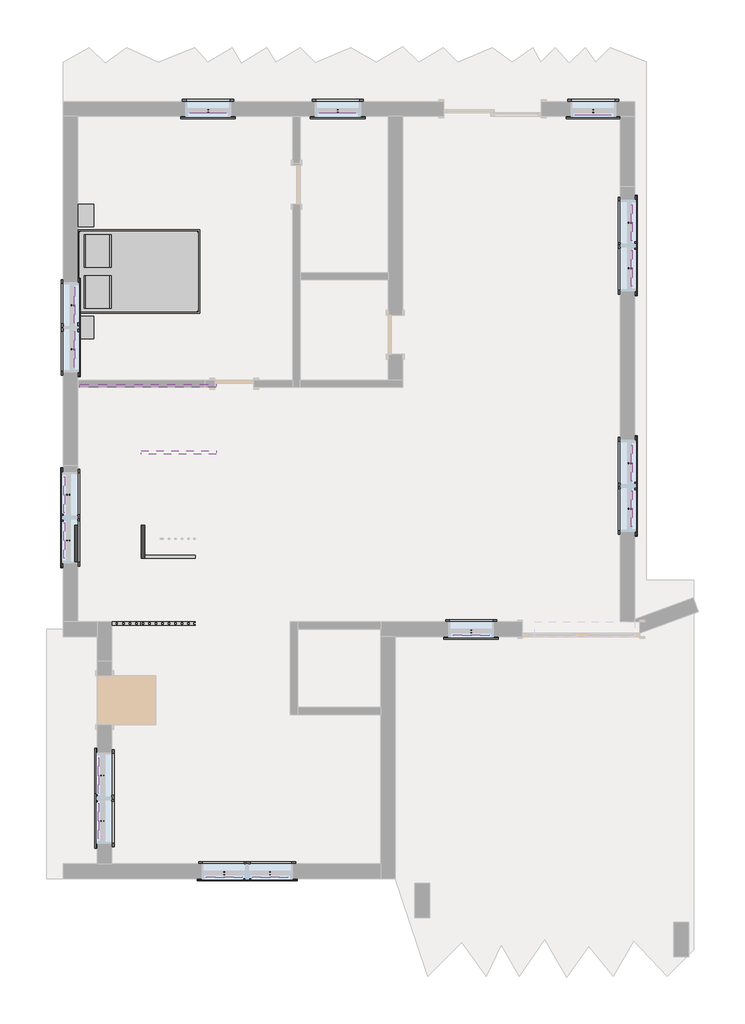
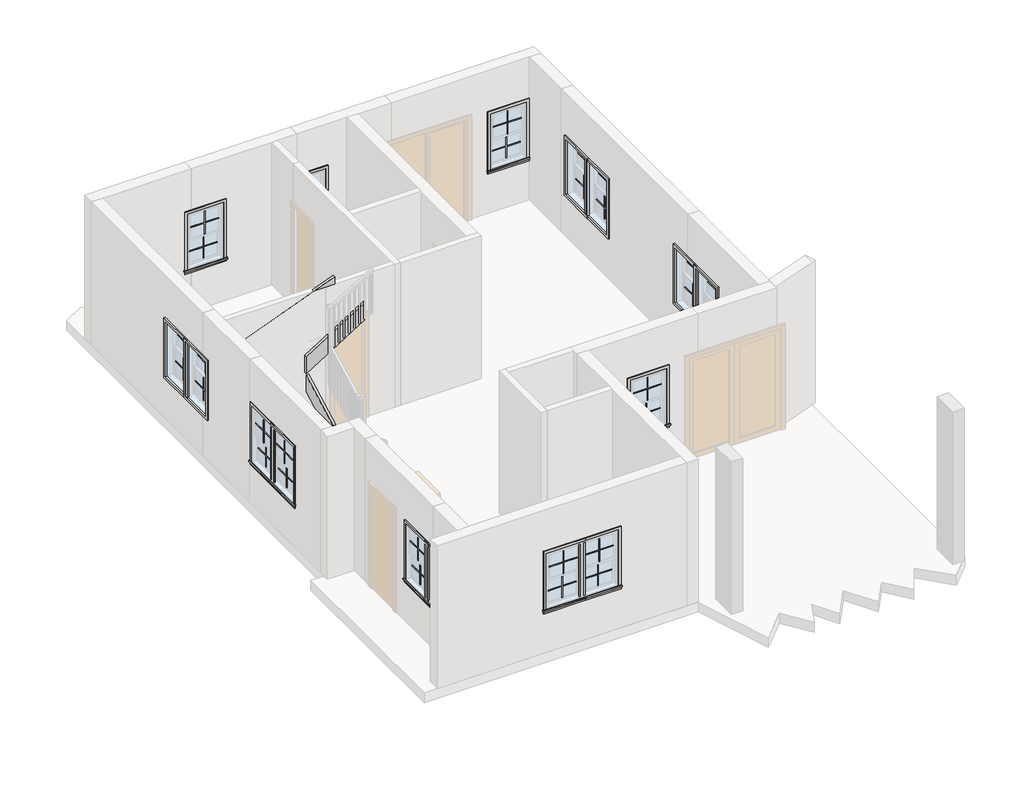
# One storey, part 3 of 3: 64 proxies, 6 members, 1 furniture element.
"""IFC4 building model written with IfcOpenShell, lengths in millimetres."""

from ifc_helpers import new_model, si_unit, frame, origin, place, context, project, spatial, polyline, outline, extrude, transform, mapped, element, save
from components import muntin_pattern_2x2_muntin_pattern_2x2_5f474966, trim_window_exterior_flat_with_sill_68241f6a, trim_window_interior_flat_picture_frame_d3d93820, modern_beds_1593_1300_x_1900_cc95cf5d

model = new_model("IFC4")

# Units and contexts
model_context = context("Model", 3, world=origin())
ifc_project = project(units=[si_unit("LENGTHUNIT", "METRE", prefix="MILLI")], contexts=[model_context])

# Site, building, storey
site = spatial("IfcSite", under=ifc_project)
building = spatial("IfcBuilding", under=site)
storey = spatial("IfcBuildingStorey", under=building, Elevation=3200.4)

# Proxies
placement = place(None, origin())
muntin_pattern_2x2_muntin_pattern_2x2_shape = muntin_pattern_2x2_muntin_pattern_2x2_5f474966(model_context)
element("IfcBuildingElementProxy", 1, Name="Muntin Pattern_2x2 : Muntin Pattern_2x2", ObjectType="Muntin Pattern_2x2 : Muntin Pattern_2x2", at=placement, inside=storey, context=model_context, shape_type="MappedRepresentation", body=[
    mapped(muntin_pattern_2x2_muntin_pattern_2x2_shape, transform((-20215.5750314, 12584.9473147, 4721.225), x_axis=(-1.0, 0.0, 0.0), y_axis=(0.0, -1.0, 0.0), z_axis=(0.0, 0.0, 1.0))),
])
element("IfcBuildingElementProxy", 2, Name="Muntin Pattern_2x2 : Muntin Pattern_2x2", ObjectType="Muntin Pattern_2x2 : Muntin Pattern_2x2", at=placement, inside=storey, context=model_context, shape_type="MappedRepresentation", body=[
    mapped(muntin_pattern_2x2_muntin_pattern_2x2_shape, transform((-20215.5750314, 12629.3973147, 4191.0), x_axis=(-1.0, 0.0, 0.0), y_axis=(0.0, -1.0, 0.0), z_axis=(0.0, 0.0, 1.0))),
])
element("IfcBuildingElementProxy", 3, Name="Muntin Pattern_2x2 : Muntin Pattern_2x2", ObjectType="Muntin Pattern_2x2 : Muntin Pattern_2x2", at=placement, inside=storey, context=model_context, shape_type="MappedRepresentation", body=[
    mapped(muntin_pattern_2x2_muntin_pattern_2x2_shape, transform((-14208.4750314, 12584.9473147, 4721.225), x_axis=(-1.0, 0.0, 0.0), y_axis=(0.0, -1.0, 0.0), z_axis=(0.0, 0.0, 1.0))),
])
element("IfcBuildingElementProxy", 4, Name="Muntin Pattern_2x2 : Muntin Pattern_2x2", ObjectType="Muntin Pattern_2x2 : Muntin Pattern_2x2", at=placement, inside=storey, context=model_context, shape_type="MappedRepresentation", body=[
    mapped(muntin_pattern_2x2_muntin_pattern_2x2_shape, transform((-14208.4750314, 12629.3973147, 4191.0), x_axis=(-1.0, 0.0, 0.0), y_axis=(0.0, -1.0, 0.0), z_axis=(0.0, 0.0, 1.0))),
])
element("IfcBuildingElementProxy", 5, Name="Muntin Pattern_2x2 : Muntin Pattern_2x2", ObjectType="Muntin Pattern_2x2 : Muntin Pattern_2x2", at=placement, inside=storey, context=model_context, shape_type="MappedRepresentation", body=[
    mapped(muntin_pattern_2x2_muntin_pattern_2x2_shape, transform((-13595.7000314, 10888.3098201, 4721.225), x_axis=(0.0, -1.0, 0.0), y_axis=(1.0, 0.0, 0.0), z_axis=(0.0, 0.0, 1.0))),
])
element("IfcBuildingElementProxy", 6, Name="Muntin Pattern_2x2 : Muntin Pattern_2x2", ObjectType="Muntin Pattern_2x2 : Muntin Pattern_2x2", at=placement, inside=storey, context=model_context, shape_type="MappedRepresentation", body=[
    mapped(muntin_pattern_2x2_muntin_pattern_2x2_shape, transform((-13640.1500314, 10888.3098201, 4191.0), x_axis=(0.0, -1.0, 0.0), y_axis=(1.0, 0.0, 0.0), z_axis=(0.0, 0.0, 1.0))),
])
element("IfcBuildingElementProxy", 7, Name="Muntin Pattern_2x2 : Muntin Pattern_2x2", ObjectType="Muntin Pattern_2x2 : Muntin Pattern_2x2", at=placement, inside=storey, context=model_context, shape_type="MappedRepresentation", body=[
    mapped(muntin_pattern_2x2_muntin_pattern_2x2_shape, transform((-13595.7000314, 10177.1098201, 4721.225), x_axis=(0.0, -1.0, 0.0), y_axis=(1.0, 0.0, 0.0), z_axis=(0.0, 0.0, 1.0))),
])
element("IfcBuildingElementProxy", 8, Name="Muntin Pattern_2x2 : Muntin Pattern_2x2", ObjectType="Muntin Pattern_2x2 : Muntin Pattern_2x2", at=placement, inside=storey, context=model_context, shape_type="MappedRepresentation", body=[
    mapped(muntin_pattern_2x2_muntin_pattern_2x2_shape, transform((-13640.1500314, 10177.1098201, 4191.0), x_axis=(0.0, -1.0, 0.0), y_axis=(1.0, 0.0, 0.0), z_axis=(0.0, 0.0, 1.0))),
])
element("IfcBuildingElementProxy", 9, Name="Muntin Pattern_2x2 : Muntin Pattern_2x2", ObjectType="Muntin Pattern_2x2 : Muntin Pattern_2x2", at=placement, inside=storey, context=model_context, shape_type="MappedRepresentation", body=[
    mapped(muntin_pattern_2x2_muntin_pattern_2x2_shape, transform((-13595.7000314, 7139.8223646, 4721.225), x_axis=(0.0, -1.0, 0.0), y_axis=(1.0, 0.0, 0.0), z_axis=(0.0, 0.0, 1.0))),
])
element("IfcBuildingElementProxy", 10, Name="Muntin Pattern_2x2 : Muntin Pattern_2x2", ObjectType="Muntin Pattern_2x2 : Muntin Pattern_2x2", at=placement, inside=storey, context=model_context, shape_type="MappedRepresentation", body=[
    mapped(muntin_pattern_2x2_muntin_pattern_2x2_shape, transform((-13640.1500314, 7139.8223646, 4191.0), x_axis=(0.0, -1.0, 0.0), y_axis=(1.0, 0.0, 0.0), z_axis=(0.0, 0.0, 1.0))),
])
element("IfcBuildingElementProxy", 11, Name="Muntin Pattern_2x2 : Muntin Pattern_2x2", ObjectType="Muntin Pattern_2x2 : Muntin Pattern_2x2", at=placement, inside=storey, context=model_context, shape_type="MappedRepresentation", body=[
    mapped(muntin_pattern_2x2_muntin_pattern_2x2_shape, transform((-13595.7000314, 6428.6223646, 4721.225), x_axis=(0.0, -1.0, 0.0), y_axis=(1.0, 0.0, 0.0), z_axis=(0.0, 0.0, 1.0))),
])
element("IfcBuildingElementProxy", 12, Name="Muntin Pattern_2x2 : Muntin Pattern_2x2", ObjectType="Muntin Pattern_2x2 : Muntin Pattern_2x2", at=placement, inside=storey, context=model_context, shape_type="MappedRepresentation", body=[
    mapped(muntin_pattern_2x2_muntin_pattern_2x2_shape, transform((-13640.1500314, 6428.6223646, 4191.0), x_axis=(0.0, -1.0, 0.0), y_axis=(1.0, 0.0, 0.0), z_axis=(0.0, 0.0, 1.0))),
])
element("IfcBuildingElementProxy", 13, Name="Muntin Pattern_2x2 : Muntin Pattern_2x2", ObjectType="Muntin Pattern_2x2 : Muntin Pattern_2x2", at=placement, inside=storey, context=model_context, shape_type="MappedRepresentation", body=[
    mapped(muntin_pattern_2x2_muntin_pattern_2x2_shape, transform((-19961.4931686, 697.7473646, 4721.225), x_axis=(-1.0, 0.0, 0.0), y_axis=(0.0, -1.0, 0.0), z_axis=(0.0, 0.0, 1.0))),
])
element("IfcBuildingElementProxy", 14, Name="Muntin Pattern_2x2 : Muntin Pattern_2x2", ObjectType="Muntin Pattern_2x2 : Muntin Pattern_2x2", at=placement, inside=storey, context=model_context, shape_type="MappedRepresentation", body=[
    mapped(muntin_pattern_2x2_muntin_pattern_2x2_shape, transform((-19961.4931686, 742.1973646, 4191.0), x_axis=(-1.0, 0.0, 0.0), y_axis=(0.0, -1.0, 0.0), z_axis=(0.0, 0.0, 1.0))),
])
element("IfcBuildingElementProxy", 15, Name="Muntin Pattern_2x2 : Muntin Pattern_2x2", ObjectType="Muntin Pattern_2x2 : Muntin Pattern_2x2", at=placement, inside=storey, context=model_context, shape_type="MappedRepresentation", body=[
    mapped(muntin_pattern_2x2_muntin_pattern_2x2_shape, transform((-19250.2931686, 697.7473646, 4721.225), x_axis=(-1.0, 0.0, 0.0), y_axis=(0.0, -1.0, 0.0), z_axis=(0.0, 0.0, 1.0))),
])
element("IfcBuildingElementProxy", 16, Name="Muntin Pattern_2x2 : Muntin Pattern_2x2", ObjectType="Muntin Pattern_2x2 : Muntin Pattern_2x2", at=placement, inside=storey, context=model_context, shape_type="MappedRepresentation", body=[
    mapped(muntin_pattern_2x2_muntin_pattern_2x2_shape, transform((-19250.2931686, 742.1973646, 4191.0), x_axis=(-1.0, 0.0, 0.0), y_axis=(0.0, -1.0, 0.0), z_axis=(0.0, 0.0, 1.0))),
])
element("IfcBuildingElementProxy", 17, Name="Muntin Pattern_2x2 : Muntin Pattern_2x2", ObjectType="Muntin Pattern_2x2 : Muntin Pattern_2x2", at=placement, inside=storey, context=model_context, shape_type="MappedRepresentation", body=[
    mapped(muntin_pattern_2x2_muntin_pattern_2x2_shape, transform((-21907.8500314, 2269.3723646, 4721.225), x_axis=(0.0, 1.0, 0.0), y_axis=(-1.0, 0.0, 0.0), z_axis=(0.0, 0.0, 1.0))),
])
element("IfcBuildingElementProxy", 18, Name="Muntin Pattern_2x2 : Muntin Pattern_2x2", ObjectType="Muntin Pattern_2x2 : Muntin Pattern_2x2", at=placement, inside=storey, context=model_context, shape_type="MappedRepresentation", body=[
    mapped(muntin_pattern_2x2_muntin_pattern_2x2_shape, transform((-21863.4000314, 2269.3723646, 4191.0), x_axis=(0.0, 1.0, 0.0), y_axis=(-1.0, 0.0, 0.0), z_axis=(0.0, 0.0, 1.0))),
])
element("IfcBuildingElementProxy", 19, Name="Muntin Pattern_2x2 : Muntin Pattern_2x2", ObjectType="Muntin Pattern_2x2 : Muntin Pattern_2x2", at=placement, inside=storey, context=model_context, shape_type="MappedRepresentation", body=[
    mapped(muntin_pattern_2x2_muntin_pattern_2x2_shape, transform((-21907.8500314, 1558.1723646, 4721.225), x_axis=(0.0, 1.0, 0.0), y_axis=(-1.0, 0.0, 0.0), z_axis=(0.0, 0.0, 1.0))),
])
element("IfcBuildingElementProxy", 20, Name="Muntin Pattern_2x2 : Muntin Pattern_2x2", ObjectType="Muntin Pattern_2x2 : Muntin Pattern_2x2", at=placement, inside=storey, context=model_context, shape_type="MappedRepresentation", body=[
    mapped(muntin_pattern_2x2_muntin_pattern_2x2_shape, transform((-21863.4000314, 1558.1723646, 4191.0), x_axis=(0.0, 1.0, 0.0), y_axis=(-1.0, 0.0, 0.0), z_axis=(0.0, 0.0, 1.0))),
])
element("IfcBuildingElementProxy", 21, Name="Muntin Pattern_2x2 : Muntin Pattern_2x2", ObjectType="Muntin Pattern_2x2 : Muntin Pattern_2x2", at=placement, inside=storey, context=model_context, shape_type="MappedRepresentation", body=[
    mapped(muntin_pattern_2x2_muntin_pattern_2x2_shape, transform((-22441.2502061, 6644.5223643, 4721.225), x_axis=(0.0, 1.0, 0.0), y_axis=(-1.0, 0.0, 0.0), z_axis=(0.0, 0.0, 1.0))),
])
element("IfcBuildingElementProxy", 22, Name="Muntin Pattern_2x2 : Muntin Pattern_2x2", ObjectType="Muntin Pattern_2x2 : Muntin Pattern_2x2", at=placement, inside=storey, context=model_context, shape_type="MappedRepresentation", body=[
    mapped(muntin_pattern_2x2_muntin_pattern_2x2_shape, transform((-22396.8002061, 6644.5223643, 4191.0), x_axis=(0.0, 1.0, 0.0), y_axis=(-1.0, 0.0, 0.0), z_axis=(0.0, 0.0, 1.0))),
])
element("IfcBuildingElementProxy", 23, Name="Muntin Pattern_2x2 : Muntin Pattern_2x2", ObjectType="Muntin Pattern_2x2 : Muntin Pattern_2x2", at=placement, inside=storey, context=model_context, shape_type="MappedRepresentation", body=[
    mapped(muntin_pattern_2x2_muntin_pattern_2x2_shape, transform((-22441.2502061, 5933.3223643, 4721.225), x_axis=(0.0, 1.0, 0.0), y_axis=(-1.0, 0.0, 0.0), z_axis=(0.0, 0.0, 1.0))),
])
element("IfcBuildingElementProxy", 24, Name="Muntin Pattern_2x2 : Muntin Pattern_2x2", ObjectType="Muntin Pattern_2x2 : Muntin Pattern_2x2", at=placement, inside=storey, context=model_context, shape_type="MappedRepresentation", body=[
    mapped(muntin_pattern_2x2_muntin_pattern_2x2_shape, transform((-22396.8002061, 5933.3223643, 4191.0), x_axis=(0.0, 1.0, 0.0), y_axis=(-1.0, 0.0, 0.0), z_axis=(0.0, 0.0, 1.0))),
])
element("IfcBuildingElementProxy", 25, Name="Muntin Pattern_2x2 : Muntin Pattern_2x2", ObjectType="Muntin Pattern_2x2 : Muntin Pattern_2x2", at=placement, inside=storey, context=model_context, shape_type="MappedRepresentation", body=[
    mapped(muntin_pattern_2x2_muntin_pattern_2x2_shape, transform((-22282.5000314, 9599.539033, 4721.225), x_axis=(0.0, -1.0, 0.0), y_axis=(1.0, 0.0, 0.0), z_axis=(0.0, 0.0, 1.0))),
])
element("IfcBuildingElementProxy", 26, Name="Muntin Pattern_2x2 : Muntin Pattern_2x2", ObjectType="Muntin Pattern_2x2 : Muntin Pattern_2x2", at=placement, inside=storey, context=model_context, shape_type="MappedRepresentation", body=[
    mapped(muntin_pattern_2x2_muntin_pattern_2x2_shape, transform((-22326.9500314, 9599.539033, 4191.0), x_axis=(0.0, -1.0, 0.0), y_axis=(1.0, 0.0, 0.0), z_axis=(0.0, 0.0, 1.0))),
])
element("IfcBuildingElementProxy", 27, Name="Muntin Pattern_2x2 : Muntin Pattern_2x2", ObjectType="Muntin Pattern_2x2 : Muntin Pattern_2x2", at=placement, inside=storey, context=model_context, shape_type="MappedRepresentation", body=[
    mapped(muntin_pattern_2x2_muntin_pattern_2x2_shape, transform((-22282.5000314, 8913.739033, 4721.225), x_axis=(0.0, -1.0, 0.0), y_axis=(1.0, 0.0, 0.0), z_axis=(0.0, 0.0, 1.0))),
])
element("IfcBuildingElementProxy", 28, Name="Muntin Pattern_2x2 : Muntin Pattern_2x2", ObjectType="Muntin Pattern_2x2 : Muntin Pattern_2x2", at=placement, inside=storey, context=model_context, shape_type="MappedRepresentation", body=[
    mapped(muntin_pattern_2x2_muntin_pattern_2x2_shape, transform((-22326.9500314, 8913.739033, 4191.0), x_axis=(0.0, -1.0, 0.0), y_axis=(1.0, 0.0, 0.0), z_axis=(0.0, 0.0, 1.0))),
])
element("IfcBuildingElementProxy", 29, Name="Muntin Pattern_2x2 : Muntin Pattern_2x2", ObjectType="Muntin Pattern_2x2 : Muntin Pattern_2x2", at=placement, inside=storey, context=model_context, shape_type="MappedRepresentation", body=[
    mapped(muntin_pattern_2x2_muntin_pattern_2x2_shape, transform((-18193.8494379, 12584.9473147, 4721.225), x_axis=(-1.0, 0.0, 0.0), y_axis=(0.0, -1.0, 0.0), z_axis=(0.0, 0.0, 1.0))),
])
element("IfcBuildingElementProxy", 30, Name="Muntin Pattern_2x2 : Muntin Pattern_2x2", ObjectType="Muntin Pattern_2x2 : Muntin Pattern_2x2", at=placement, inside=storey, context=model_context, shape_type="MappedRepresentation", body=[
    mapped(muntin_pattern_2x2_muntin_pattern_2x2_shape, transform((-18193.8494379, 12629.3973147, 4191.0), x_axis=(-1.0, 0.0, 0.0), y_axis=(0.0, -1.0, 0.0), z_axis=(0.0, 0.0, 1.0))),
])
element("IfcBuildingElementProxy", 31, Name="Muntin Pattern_2x2 : Muntin Pattern_2x2", ObjectType="Muntin Pattern_2x2 : Muntin Pattern_2x2", at=placement, inside=storey, context=model_context, shape_type="MappedRepresentation", body=[
    mapped(muntin_pattern_2x2_muntin_pattern_2x2_shape, transform((-16113.4750314, 4469.6473722, 4721.225), x_axis=(-1.0, 0.0, 0.0), y_axis=(0.0, -1.0, 0.0), z_axis=(0.0, 0.0, 1.0))),
])
element("IfcBuildingElementProxy", 32, Name="Muntin Pattern_2x2 : Muntin Pattern_2x2", ObjectType="Muntin Pattern_2x2 : Muntin Pattern_2x2", at=placement, inside=storey, context=model_context, shape_type="MappedRepresentation", body=[
    mapped(muntin_pattern_2x2_muntin_pattern_2x2_shape, transform((-16113.4750314, 4514.0973722, 4191.0), x_axis=(-1.0, 0.0, 0.0), y_axis=(0.0, -1.0, 0.0), z_axis=(0.0, 0.0, 1.0))),
])
trim_window_exterior_flat_with_sill_shape = trim_window_exterior_flat_with_sill_68241f6a(model_context)
element("IfcBuildingElementProxy", 33, Name="Trim-Window-Exterior-Flat : with Sill", ObjectType="Trim-Window-Exterior-Flat : with Sill", at=placement, inside=storey, context=model_context, shape_type="MappedRepresentation", body=[
    mapped(trim_window_exterior_flat_with_sill_shape, transform((-20215.5750314, 12550.0223147, 5283.2), x_axis=(1.0, 0.0, 0.0), y_axis=(0.0, 0.0, 1.0), z_axis=(0.0, -1.0, 0.0))),
])
element("IfcBuildingElementProxy", 34, Name="Trim-Window-Exterior-Flat : with Sill", ObjectType="Trim-Window-Exterior-Flat : with Sill", at=placement, inside=storey, context=model_context, shape_type="MappedRepresentation", body=[
    mapped(trim_window_exterior_flat_with_sill_shape, transform((-14208.4750314, 12550.0223147, 5283.2), x_axis=(1.0, 0.0, 0.0), y_axis=(0.0, 0.0, 1.0), z_axis=(0.0, -1.0, 0.0))),
])
element("IfcBuildingElementProxy", 35, Name="Trim-Window-Exterior-Flat : with Sill", ObjectType="Trim-Window-Exterior-Flat : with Sill", at=placement, inside=storey, context=model_context, shape_type="MappedRepresentation", body=[
    mapped(trim_window_exterior_flat_with_sill_shape, transform((-13560.7750314, 10888.3098201, 5283.2), x_axis=(0.0, 1.0, 0.0), y_axis=(0.0, 0.0, 1.0), z_axis=(1.0, 0.0, 0.0))),
])
element("IfcBuildingElementProxy", 36, Name="Trim-Window-Exterior-Flat : with Sill", ObjectType="Trim-Window-Exterior-Flat : with Sill", at=placement, inside=storey, context=model_context, shape_type="MappedRepresentation", body=[
    mapped(trim_window_exterior_flat_with_sill_shape, transform((-13560.7750314, 10177.1098201, 5283.2), x_axis=(0.0, 1.0, 0.0), y_axis=(0.0, 0.0, 1.0), z_axis=(1.0, 0.0, 0.0))),
])
element("IfcBuildingElementProxy", 37, Name="Trim-Window-Exterior-Flat : with Sill", ObjectType="Trim-Window-Exterior-Flat : with Sill", at=placement, inside=storey, context=model_context, shape_type="MappedRepresentation", body=[
    mapped(trim_window_exterior_flat_with_sill_shape, transform((-13560.7750314, 7139.8223646, 5283.2), x_axis=(0.0, 1.0, 0.0), y_axis=(0.0, 0.0, 1.0), z_axis=(1.0, 0.0, 0.0))),
])
element("IfcBuildingElementProxy", 38, Name="Trim-Window-Exterior-Flat : with Sill", ObjectType="Trim-Window-Exterior-Flat : with Sill", at=placement, inside=storey, context=model_context, shape_type="MappedRepresentation", body=[
    mapped(trim_window_exterior_flat_with_sill_shape, transform((-13560.7750314, 6428.6223646, 5283.2), x_axis=(0.0, 1.0, 0.0), y_axis=(0.0, 0.0, 1.0), z_axis=(1.0, 0.0, 0.0))),
])
element("IfcBuildingElementProxy", 39, Name="Trim-Window-Exterior-Flat : with Sill", ObjectType="Trim-Window-Exterior-Flat : with Sill", at=placement, inside=storey, context=model_context, shape_type="MappedRepresentation", body=[
    mapped(trim_window_exterior_flat_with_sill_shape, transform((-19961.4931686, 662.8223646, 5283.2), x_axis=(1.0, 0.0, 0.0), y_axis=(0.0, 0.0, 1.0), z_axis=(0.0, -1.0, 0.0))),
])
element("IfcBuildingElementProxy", 40, Name="Trim-Window-Exterior-Flat : with Sill", ObjectType="Trim-Window-Exterior-Flat : with Sill", at=placement, inside=storey, context=model_context, shape_type="MappedRepresentation", body=[
    mapped(trim_window_exterior_flat_with_sill_shape, transform((-19250.2931686, 662.8223646, 5283.2), x_axis=(1.0, 0.0, 0.0), y_axis=(0.0, 0.0, 1.0), z_axis=(0.0, -1.0, 0.0))),
])
element("IfcBuildingElementProxy", 41, Name="Trim-Window-Exterior-Flat : with Sill", ObjectType="Trim-Window-Exterior-Flat : with Sill", at=placement, inside=storey, context=model_context, shape_type="MappedRepresentation", body=[
    mapped(trim_window_exterior_flat_with_sill_shape, transform((-21942.7750314, 2269.3723646, 5283.2), x_axis=(0.0, -1.0, 0.0), y_axis=(0.0, 0.0, 1.0), z_axis=(-1.0, 0.0, 0.0))),
])
element("IfcBuildingElementProxy", 42, Name="Trim-Window-Exterior-Flat : with Sill", ObjectType="Trim-Window-Exterior-Flat : with Sill", at=placement, inside=storey, context=model_context, shape_type="MappedRepresentation", body=[
    mapped(trim_window_exterior_flat_with_sill_shape, transform((-21942.7750314, 1558.1723646, 5283.2), x_axis=(0.0, -1.0, 0.0), y_axis=(0.0, 0.0, 1.0), z_axis=(-1.0, 0.0, 0.0))),
])
element("IfcBuildingElementProxy", 43, Name="Trim-Window-Exterior-Flat : with Sill", ObjectType="Trim-Window-Exterior-Flat : with Sill", at=placement, inside=storey, context=model_context, shape_type="MappedRepresentation", body=[
    mapped(trim_window_exterior_flat_with_sill_shape, transform((-22476.1752061, 6644.5223643, 5283.2), x_axis=(0.0, -1.0, 0.0), y_axis=(0.0, 0.0, 1.0), z_axis=(-1.0, 0.0, 0.0))),
])
element("IfcBuildingElementProxy", 44, Name="Trim-Window-Exterior-Flat : with Sill", ObjectType="Trim-Window-Exterior-Flat : with Sill", at=placement, inside=storey, context=model_context, shape_type="MappedRepresentation", body=[
    mapped(trim_window_exterior_flat_with_sill_shape, transform((-22476.1752061, 5933.3223643, 5283.2), x_axis=(0.0, -1.0, 0.0), y_axis=(0.0, 0.0, 1.0), z_axis=(-1.0, 0.0, 0.0))),
])
element("IfcBuildingElementProxy", 45, Name="Trim-Window-Exterior-Flat : with Sill", ObjectType="Trim-Window-Exterior-Flat : with Sill", at=placement, inside=storey, context=model_context, shape_type="MappedRepresentation", body=[
    mapped(trim_window_exterior_flat_with_sill_shape, transform((-22247.5750314, 9599.539033, 5283.2), x_axis=(0.0, 1.0, 0.0), y_axis=(0.0, 0.0, 1.0), z_axis=(1.0, 0.0, 0.0))),
])
element("IfcBuildingElementProxy", 46, Name="Trim-Window-Exterior-Flat : with Sill", ObjectType="Trim-Window-Exterior-Flat : with Sill", at=placement, inside=storey, context=model_context, shape_type="MappedRepresentation", body=[
    mapped(trim_window_exterior_flat_with_sill_shape, transform((-22247.5750314, 8913.739033, 5283.2), x_axis=(0.0, 1.0, 0.0), y_axis=(0.0, 0.0, 1.0), z_axis=(1.0, 0.0, 0.0))),
])
element("IfcBuildingElementProxy", 47, Name="Trim-Window-Exterior-Flat : with Sill", ObjectType="Trim-Window-Exterior-Flat : with Sill", at=placement, inside=storey, context=model_context, shape_type="MappedRepresentation", body=[
    mapped(trim_window_exterior_flat_with_sill_shape, transform((-18193.8494379, 12550.0223147, 5283.2), x_axis=(1.0, 0.0, 0.0), y_axis=(0.0, 0.0, 1.0), z_axis=(0.0, -1.0, 0.0))),
])
element("IfcBuildingElementProxy", 48, Name="Trim-Window-Exterior-Flat : with Sill", ObjectType="Trim-Window-Exterior-Flat : with Sill", at=placement, inside=storey, context=model_context, shape_type="MappedRepresentation", body=[
    mapped(trim_window_exterior_flat_with_sill_shape, transform((-16113.4750314, 4434.7223722, 5283.2), x_axis=(1.0, 0.0, 0.0), y_axis=(0.0, 0.0, 1.0), z_axis=(0.0, -1.0, 0.0))),
])
trim_window_interior_flat_picture_frame_shape = trim_window_interior_flat_picture_frame_d3d93820(model_context)
element("IfcBuildingElementProxy", 49, Name="Trim-Window-Interior-Flat : Picture Frame", ObjectType="Trim-Window-Interior-Flat : Picture Frame", at=placement, inside=storey, context=model_context, shape_type="MappedRepresentation", body=[
    mapped(trim_window_interior_flat_picture_frame_shape, transform((-20215.5750314, 12778.6223147, 5283.2), x_axis=(-1.0, 0.0, 0.0), y_axis=(0.0, 0.0, 1.0), z_axis=(0.0, 1.0, 0.0))),
])
element("IfcBuildingElementProxy", 50, Name="Trim-Window-Interior-Flat : Picture Frame", ObjectType="Trim-Window-Interior-Flat : Picture Frame", at=placement, inside=storey, context=model_context, shape_type="MappedRepresentation", body=[
    mapped(trim_window_interior_flat_picture_frame_shape, transform((-14208.4750314, 12778.6223147, 5283.2), x_axis=(-1.0, 0.0, 0.0), y_axis=(0.0, 0.0, 1.0), z_axis=(0.0, 1.0, 0.0))),
])
element("IfcBuildingElementProxy", 51, Name="Trim-Window-Interior-Flat : Picture Frame", ObjectType="Trim-Window-Interior-Flat : Picture Frame", at=placement, inside=storey, context=model_context, shape_type="MappedRepresentation", body=[
    mapped(trim_window_interior_flat_picture_frame_shape, transform((-13789.3750314, 10888.3098201, 5283.2), x_axis=(0.0, -1.0, 0.0), y_axis=(0.0, 0.0, 1.0), z_axis=(-1.0, 0.0, 0.0))),
])
element("IfcBuildingElementProxy", 52, Name="Trim-Window-Interior-Flat : Picture Frame", ObjectType="Trim-Window-Interior-Flat : Picture Frame", at=placement, inside=storey, context=model_context, shape_type="MappedRepresentation", body=[
    mapped(trim_window_interior_flat_picture_frame_shape, transform((-13789.3750314, 10177.1098201, 5283.2), x_axis=(0.0, -1.0, 0.0), y_axis=(0.0, 0.0, 1.0), z_axis=(-1.0, 0.0, 0.0))),
])
element("IfcBuildingElementProxy", 53, Name="Trim-Window-Interior-Flat : Picture Frame", ObjectType="Trim-Window-Interior-Flat : Picture Frame", at=placement, inside=storey, context=model_context, shape_type="MappedRepresentation", body=[
    mapped(trim_window_interior_flat_picture_frame_shape, transform((-13789.3750314, 7139.8223646, 5283.2), x_axis=(0.0, -1.0, 0.0), y_axis=(0.0, 0.0, 1.0), z_axis=(-1.0, 0.0, 0.0))),
])
element("IfcBuildingElementProxy", 54, Name="Trim-Window-Interior-Flat : Picture Frame", ObjectType="Trim-Window-Interior-Flat : Picture Frame", at=placement, inside=storey, context=model_context, shape_type="MappedRepresentation", body=[
    mapped(trim_window_interior_flat_picture_frame_shape, transform((-13789.3750314, 6428.6223646, 5283.2), x_axis=(0.0, -1.0, 0.0), y_axis=(0.0, 0.0, 1.0), z_axis=(-1.0, 0.0, 0.0))),
])
element("IfcBuildingElementProxy", 55, Name="Trim-Window-Interior-Flat : Picture Frame", ObjectType="Trim-Window-Interior-Flat : Picture Frame", at=placement, inside=storey, context=model_context, shape_type="MappedRepresentation", body=[
    mapped(trim_window_interior_flat_picture_frame_shape, transform((-19961.4931686, 891.4223646, 5283.2), x_axis=(-1.0, 0.0, 0.0), y_axis=(0.0, 0.0, 1.0), z_axis=(0.0, 1.0, 0.0))),
])
element("IfcBuildingElementProxy", 56, Name="Trim-Window-Interior-Flat : Picture Frame", ObjectType="Trim-Window-Interior-Flat : Picture Frame", at=placement, inside=storey, context=model_context, shape_type="MappedRepresentation", body=[
    mapped(trim_window_interior_flat_picture_frame_shape, transform((-19250.2931686, 891.4223646, 5283.2), x_axis=(-1.0, 0.0, 0.0), y_axis=(0.0, 0.0, 1.0), z_axis=(0.0, 1.0, 0.0))),
])
element("IfcBuildingElementProxy", 57, Name="Trim-Window-Interior-Flat : Picture Frame", ObjectType="Trim-Window-Interior-Flat : Picture Frame", at=placement, inside=storey, context=model_context, shape_type="MappedRepresentation", body=[
    mapped(trim_window_interior_flat_picture_frame_shape, transform((-21714.1750314, 2269.3723646, 5283.2), x_axis=(0.0, 1.0, 0.0), y_axis=(0.0, 0.0, 1.0), z_axis=(1.0, 0.0, 0.0))),
])
element("IfcBuildingElementProxy", 58, Name="Trim-Window-Interior-Flat : Picture Frame", ObjectType="Trim-Window-Interior-Flat : Picture Frame", at=placement, inside=storey, context=model_context, shape_type="MappedRepresentation", body=[
    mapped(trim_window_interior_flat_picture_frame_shape, transform((-21714.1750314, 1558.1723646, 5283.2), x_axis=(0.0, 1.0, 0.0), y_axis=(0.0, 0.0, 1.0), z_axis=(1.0, 0.0, 0.0))),
])
element("IfcBuildingElementProxy", 59, Name="Trim-Window-Interior-Flat : Picture Frame", ObjectType="Trim-Window-Interior-Flat : Picture Frame", at=placement, inside=storey, context=model_context, shape_type="MappedRepresentation", body=[
    mapped(trim_window_interior_flat_picture_frame_shape, transform((-22247.5752061, 6644.5223643, 5283.2), x_axis=(0.0, 1.0, 0.0), y_axis=(0.0, 0.0, 1.0), z_axis=(1.0, 0.0, 0.0))),
])
element("IfcBuildingElementProxy", 60, Name="Trim-Window-Interior-Flat : Picture Frame", ObjectType="Trim-Window-Interior-Flat : Picture Frame", at=placement, inside=storey, context=model_context, shape_type="MappedRepresentation", body=[
    mapped(trim_window_interior_flat_picture_frame_shape, transform((-22247.5752061, 5933.3223643, 5283.2), x_axis=(0.0, 1.0, 0.0), y_axis=(0.0, 0.0, 1.0), z_axis=(1.0, 0.0, 0.0))),
])
element("IfcBuildingElementProxy", 61, Name="Trim-Window-Interior-Flat : Picture Frame", ObjectType="Trim-Window-Interior-Flat : Picture Frame", at=placement, inside=storey, context=model_context, shape_type="MappedRepresentation", body=[
    mapped(trim_window_interior_flat_picture_frame_shape, transform((-22476.1750314, 9599.539033, 5283.2), x_axis=(0.0, -1.0, 0.0), y_axis=(0.0, 0.0, 1.0), z_axis=(-1.0, 0.0, 0.0))),
])
element("IfcBuildingElementProxy", 62, Name="Trim-Window-Interior-Flat : Picture Frame", ObjectType="Trim-Window-Interior-Flat : Picture Frame", at=placement, inside=storey, context=model_context, shape_type="MappedRepresentation", body=[
    mapped(trim_window_interior_flat_picture_frame_shape, transform((-22476.1750314, 8913.739033, 5283.2), x_axis=(0.0, -1.0, 0.0), y_axis=(0.0, 0.0, 1.0), z_axis=(-1.0, 0.0, 0.0))),
])
element("IfcBuildingElementProxy", 63, Name="Trim-Window-Interior-Flat : Picture Frame", ObjectType="Trim-Window-Interior-Flat : Picture Frame", at=placement, inside=storey, context=model_context, shape_type="MappedRepresentation", body=[
    mapped(trim_window_interior_flat_picture_frame_shape, transform((-18193.8494379, 12778.6223147, 5283.2), x_axis=(-1.0, 0.0, 0.0), y_axis=(0.0, 0.0, 1.0), z_axis=(0.0, 1.0, 0.0))),
])
element("IfcBuildingElementProxy", 64, Name="Trim-Window-Interior-Flat : Picture Frame", ObjectType="Trim-Window-Interior-Flat : Picture Frame", at=placement, inside=storey, context=model_context, shape_type="MappedRepresentation", body=[
    mapped(trim_window_interior_flat_picture_frame_shape, transform((-16113.4750314, 4663.3223722, 5283.2), x_axis=(-1.0, 0.0, 0.0), y_axis=(0.0, 0.0, 1.0), z_axis=(0.0, 1.0, 0.0))),
])

# Furniture
modern_beds_1593_1300_x_1900_shape = modern_beds_1593_1300_x_1900_cc95cf5d(model_context)
element("IfcFurniture", 65, ObjectType="Modern_Beds_1593 : 1300 x 1900", at=placement, inside=storey, context=model_context, shape_type="MappedRepresentation", body=[
    mapped(modern_beds_1593_1300_x_1900_shape, transform((-21532.0045396, 9789.8241008, 3200.4), x_axis=(0.0, 1.0, 0.0), y_axis=(-1.0, 0.0, 0.0), z_axis=(0.0, 0.0, 1.0))),
])

# Members
element("IfcMember", 66, ObjectType="Stringer - 2\" Width", at=placement, inside=storey, context=model_context, shape_type="SweptSolid", body=[
    extrude(outline(polyline([(3330.9252239, -20418.7750314), (3653.2815263, -20418.7750314), (3947.3746925, -21273.045657), (3947.3746925, -22209.4139641), (3330.9252239, -20418.7750314)])), frame((0.0, 4612.5223646, 0.0), z_axis=(0.0, 1.0, 0.0), x_axis=(0.0, 0.0, 1.0)), (0.0, 0.0, 1.0), 50.8),
])
element("IfcMember", 67, ObjectType="Stringer - 2\" Width", at=placement, inside=storey, context=model_context, shape_type="SweptSolid", body=[
    extrude(outline(polyline([(4688.0958922, 3960.5121693), (7646.6888829, 5529.4629977), (8297.2722107, 5529.4629977), (5338.67922, 3960.5121693), (4688.0958922, 3960.5121693)])), frame((-22298.3752061, 0.0, 0.0), z_axis=(1.0, 0.0, 0.0), x_axis=(0.0, 1.0, 0.0)), (0.0, 0.0, 1.0), 50.8),
])
element("IfcMember", 68, ObjectType="Stringer - 2\" Width", at=placement, inside=storey, context=model_context, shape_type="SweptSolid", body=[
    extrude(outline(polyline([(5542.004746, -21363.7701417), (6031.1206787, -20088.5750314), (6357.5726538, -20088.5750314), (5542.004746, -22214.8770766), (5542.004746, -21363.7701417)])), frame((0.0, 8320.9223646, 0.0), z_axis=(0.0, 1.0, 0.0), x_axis=(0.0, 0.0, 1.0)), (0.0, 0.0, 1.0), 50.8),
])
element("IfcMember", 69, ObjectType="Stringer - 2\" Width", at=placement, inside=storey, context=model_context, shape_type="SweptSolid", body=[
    extrude(outline(polyline([(3231.9282995, -20418.7750314), (3593.2106437, -20418.7750314), (4094.283371, -21206.1750314), (3733.0010268, -21206.1750314), (3231.9282995, -20418.7750314)])), frame((0.0, 5653.9223646, 0.0), z_axis=(0.0, 1.0, 0.0), x_axis=(0.0, 0.0, 1.0)), (0.0, 0.0, 1.0), 50.8),
])
element("IfcMember", 70, ObjectType="Stringer - 2\" Width", at=placement, inside=storey, context=model_context, shape_type="SweptSolid", body=[
    extrude(outline(polyline([(5653.9223646, 4127.6865642), (5653.9223646, 4472.6928743), (7279.5223646, 5334.7534804), (7279.5223646, 4989.7471702), (5653.9223646, 4127.6865642)])), frame((-21256.9750314, 0.0, 0.0), z_axis=(1.0, 0.0, 0.0), x_axis=(0.0, 1.0, 0.0)), (0.0, 0.0, 1.0), 50.8),
])
element("IfcMember", 71, ObjectType="Stringer - 2\" Width", at=placement, inside=storey, context=model_context, shape_type="SweptSolid", body=[
    extrude(outline(polyline([(5725.0057942, -21256.9750314), (5366.7538932, -21256.9750314), (6088.4127167, -20088.5750314), (6446.6646178, -20088.5750314), (5725.0057942, -21256.9750314)])), frame((0.0, 7279.5223646, 0.0), z_axis=(0.0, 1.0, 0.0), x_axis=(0.0, 0.0, 1.0)), (0.0, 0.0, 1.0), 50.8),
])

save(model, "model.ifc")

# Revit data of these elements
# Type "Muntin Pattern_2x2 : Muntin Pattern_2x2"
#   Width [instance default] = 4' - 0"
#   Thickness = 0' - 0 1/2"
#   Height [instance default] = 4' - 0"
#   Distance = 0' - 0 3/4"
#   Interior Material [instance default] = none
#   Exterior Material [instance default] = none
#   Default Elevation = 0
# Type "Trim-Window-Exterior-Flat : with Sill"
#   Trim Width = 0' - 2 1/4"
#   Trim Thickness_Picture Frame = 0' - 1 1/4"
#   Trim Thickness_with Sill = 0' - 0 3/4"
#   Sill Thickness = 0' - 1 1/4"
#   Opening Width [instance default] = 2' - 0"
#   Opening Height [instance default] = 3' - 0"
#   Default Elevation = 4' - 0"
#   Sill = yes
#   Picture Frame = no
#   Trim Material [instance default] = none
# Type "Trim-Window-Interior-Flat : Picture Frame"
#   Trim Thickness_Picture Frame = 0' - 1 1/4"
#   Trim Width = 0' - 2 1/4"
#   Trim Thickness_with Sill = 0' - 0 3/4"
#   Sill Thickness = 0' - 1 1/4"
#   Opening Width [instance default] = 2' - 0"
#   Opening Height [instance default] = 3' - 0"
#   Default Elevation = 4' - 0"
#   Sill = no
#   Picture Frame = yes
#   Trim Material [instance default] = none
# Type "Modern_Beds_1593 : 1300 x 1900"
#   Length = 6' - 2.80315"
#   Width = 4' - 3.1811"
#   Frame Material = Bed-Wood
#   Mattress Material = Bed-Cover
#   Default Elevation = 0
# Elements 1, 2, 3, 4, 5, 6, 7, 8, 9, 10, 11, 12, 13, 14, 15, 16, 17, 18, 19, 20, 21, 22, 23, 24, 25, 26, 27, 28, 29, 30, 31, 32 (IfcBuildingElementProxy, "Muntin Pattern_2x2 : Muntin Pattern_2x2")
#   Width = 1' - 10"
#   Height = 1' - 7 1/8"
#   Interior Material = Wood - Stained
#   Exterior Material = Clad - White
#   Phase Created = New Construction
#   Materials on its faces: "Clad - White", "Wood - Stained"
# Elements 33, 34, 35, 36, 37, 38, 39, 40, 41, 42, 43, 44, 45, 46, 47, 48 (IfcBuildingElementProxy, "Trim-Window-Exterior-Flat : with Sill")
#   Opening Width = 2' - 4"
#   Opening Height = 3' - 10"
#   Trim Material = Clad - White
#   Phase Created = New Construction
#   Materials on its faces: "Clad - White"
# Elements 49, 50, 51, 52, 53, 54, 55, 56, 57, 58, 59, 60, 61, 62, 63, 64 (IfcBuildingElementProxy, "Trim-Window-Interior-Flat : Picture Frame")
#   Opening Width = 2' - 4"
#   Opening Height = 3' - 10"
#   Trim Material = Wood - Stained
#   Phase Created = New Construction
#   Materials on its faces: "Wood - Stained"
# Element 65 (IfcFurniture, "Modern_Beds_1593 : 1300 x 1900")
#   Phase Created = New Construction
#   Materials on its faces: "Bed-Metal", "Bed-Cover", "Bed-Wood"
# Elements 66, 67, 68, 69, 70, 71 (IfcMember, "Stringer - 2\" Width")
#   Phase Created = New Construction
# Materials
#   "Bed-Wood": colour RGB 224 178 126, transparency 0
#   "Bed-Cover": colour RGB 255 255 255, transparency 0
#   "Clad - White": class "Wood", colour RGB 242 242 238, transparency 0, Cost = 0
#   "Wood - Stained": class "Wood", colour RGB 224 178 126, transparency 0, Cost = 0
#   "Bed-Metal": colour RGB 247 247 247, transparency 0
